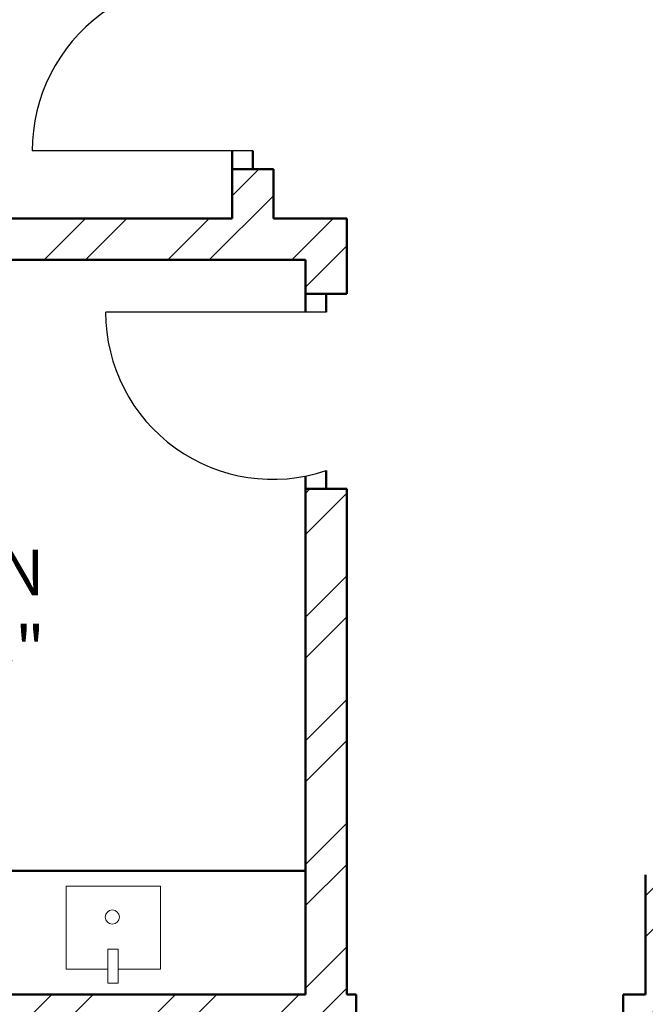
# Model space of a CAD drawing. Units: inches. Extents: x 1901 to 2863, y 888 to 2433.
# Tile 8 of 91: x 2086 to 2154, y 1442 to 1549. Entities that reach past the tile are written whole.
import ezdxf

# ---------------------------------------------------------------- set-up
doc = ezdxf.new("R2010")
doc.units = ezdxf.units.IN
for name, color, linetype, lineweight in [('A-AREA-IDEN', 7, 'Continuous', 18), ('A-DOOR', 4, 'Continuous', 25), ('A-FLOR-FIXT', 9, 'Continuous', 18), ('A-WALL', 7, 'Continuous', 50), ('A-WALL-PATT', 8, 'Continuous', 13)]:
    doc.layers.add(name, color=color, linetype=linetype, lineweight=lineweight)
doc.styles.get("Standard").update_dxf_attribs({"font": 'arial.ttf'})

msp = doc.modelspace()

# ---------------------------------------------------------------- hatches: boundary and pattern name
at = {"layer": 'A-WALL-PATT'}
h = msp.add_hatch(dxfattribs=at)
h.set_pattern_fill('ANSI32', color=256)
h.paths.add_polyline_path([(2192.5, 2274.13), (2141.26, 2274.13), (2141.26, 2269.63), (2192.5, 2269.63)])
h.paths.add_polyline_path([(2259.93, 2274.13), (2216.5, 2274.13), (2216.5, 2269.63), (2255.43, 2269.63), (2255.43, 2214.63), (2250.81, 2214.63), (2250.81, 2210.13), (2259.93, 2210.13), (2259.93, 2215.13), (2271.76, 2215.13), (2271.76, 2217.38), (2271.76, 2219.63), (2259.93, 2219.63)])
h.paths.add_polyline_path([(2171.43, 2269.63), (2166.93, 2269.63), (2166.93, 2219.63), (2121.24, 2219.63), (2121.24, 2215.13), (2166.93, 2215.13), (2166.93, 2083.13), (2161.81, 2083.13), (2161.81, 2078.63), (2171.43, 2078.63), (2177, 2078.63), (2177, 2080.88), (2177, 2083.13), (2171.43, 2083.13), (2171.43, 2210.13), (2230.91, 2210.13), (2230.91, 2212.38), (2230.91, 2214.63), (2171.43, 2214.63)])
h.paths.add_polyline_path([(2117.26, 2274.13), (2089.43, 2274.13), (2089.43, 2219.63), (2081.14, 2219.63), (2081.14, 2215.13), (2089.43, 2215.13), (2098, 2215.13), (2098, 2217.38), (2098, 2219.63), (2093.93, 2219.63), (2093.93, 2269.63), (2117.26, 2269.63), (2117.26, 2271.88)])
h.paths.add_polyline_path([(2343.43, 2219.63), (2329.29, 2219.63), (2329.29, 2215.13), (2338.93, 2215.13), (2338.93, 2184.74), (2343.43, 2184.74)])
h.paths.add_polyline_path([(2338.93, 2083.13), (2329.29, 2083.13), (2208.97, 2083.13), (2208.97, 2078.63), (2338.93, 2078.63)])
h.paths.add_polyline_path([(2343.43, 2136.74), (2338.93, 2136.74), (2338.93, 1872.63), (2343.43, 1872.63)])
h.paths.add_polyline_path([(2343.43, 1863.63), (2397.68, 1863.63), (2397.68, 1821.63), (2384.14, 1821.63), (2384.14, 1812.63), (2418.33, 1812.63), (2418.33, 1817.13), (2418.33, 1821.63), (2406.68, 1821.63), (2406.68, 1863.63), (2459.5, 1863.63), (2459.5, 1821.63), (2447.14, 1821.63), (2447.14, 1812.63), (2459.5, 1812.63), (2468.5, 1812.63), (2468.5, 1872.63), (2394.43, 1872.63), (2334.43, 1872.63), (2334.43, 1812.63), (2343.43, 1812.63), (2353.25, 1812.63), (2353.25, 1821.63), (2343.43, 1821.63)])
h.paths.add_polyline_path([(2510.01, 1872.63), (2468.5, 1872.63), (2468.5, 1868.13), (2510.01, 1868.13)])
h.paths.add_polyline_path([(2514.01, 1817.13), (2468.5, 1817.13), (2468.5, 1812.63), (2482.11, 1812.63), (2482.11, 1800.61), (2486.61, 1800.61), (2486.61, 1812.63), (2514.01, 1812.63)])
h.paths.add_polyline_path([(2299.25, 1814.88), (2299.25, 1817.13), (2295.93, 1817.13), (2295.93, 1854.17), (2293.68, 1854.17), (2291.43, 1854.17), (2291.43, 1817.13), (2266.11, 1817.13), (2266.11, 1812.63), (2299.25, 1812.63)])
h.paths.add_polyline_path([(2218.11, 1817.13), (2206.46, 1817.13), (2171.43, 1817.13), (2171.43, 1949.13), (2190.1, 1949.13), (2190.1, 1953.63), (2163.47, 1953.63), (2163.47, 1949.13), (2166.93, 1949.13), (2166.93, 1817.13), (2114.3, 1817.13), (2114.3, 1812.63), (2218.11, 1812.63)])
h.paths.add_polyline_path([(2029.43, 1970.92), (2024.93, 1970.92), (2024.93, 1912.72), (2029.43, 1912.72)])
h.paths.add_polyline_path([(2132.3, 1953.63), (2113.93, 1953.63), (2113.93, 1975.89), (2111.68, 1975.89), (2109.43, 1975.89), (2109.43, 1953.63), (2029.43, 1953.63), (2029.43, 1949.13), (2132.3, 1949.13)])
h.paths.add_polyline_path([(2029.43, 1853.61), (2029.31, 1853.61), (2029.31, 1853.61), (2029.43, 1853.61), (2029.43, 1864.72), (2024.93, 1864.72), (2024.93, 1812.63), (2066.3, 1812.63), (2066.3, 1814.88), (2066.3, 1817.13), (2029.43, 1817.13)])
h.paths.add_polyline_path([(2122.93, 2010.09), (2120.68, 2010.09), (2118.43, 2010.09), (2118.43, 2006.13), (2029.43, 2006.13), (2029.43, 2001.63), (2109.43, 2001.63), (2109.43, 1998.04), (2113.93, 1998.04), (2113.93, 2001.63), (2122.93, 2001.63)])
h.paths.add_polyline_path([(2029.43, 2031.38), (2024.93, 2031.38), (2024.93, 1994.92), (2027.18, 1994.92), (2029.43, 1994.92)])
h.paths.add_polyline_path([(2029.43, 2136.74), (2024.93, 2136.74), (2024.93, 2067.38), (2027.18, 2067.38), (2029.43, 2067.38)])
h.paths.add_polyline_path([(2125.62, 2083.13), (2029.43, 2083.13), (2029.43, 2078.63), (2118.43, 2078.63), (2118.43, 2030.71), (2122.93, 2030.71), (2122.93, 2078.63), (2125.62, 2078.63)])
h.paths.add_polyline_path([(2029.43, 2215.13), (2040.47, 2215.13), (2040.47, 2217.38), (2040.47, 2219.63), (2024.93, 2219.63), (2024.93, 2184.74), (2029.43, 2184.74), (2029.43, 2187.78)])
h.paths.add_polyline_path([(2686.43, 2274.13), (2659.28, 2274.13), (2659.28, 2269.63), (2681.93, 2269.63), (2681.93, 2219.63), (2676.82, 2219.63), (2676.82, 2215.13), (2681.93, 2215.13), (2697.01, 2215.13), (2697.01, 2217.38), (2697.01, 2219.63), (2686.43, 2219.63)])
h.paths.add_polyline_path([(2609.93, 2269.63), (2635.28, 2269.63), (2635.28, 2274.13), (2571.43, 2274.13), (2571.43, 2269.63), (2605.43, 2269.63), (2605.43, 2214.63), (2549.1, 2214.63), (2549.1, 2210.13), (2605.43, 2210.13), (2605.43, 2083.13), (2601.01, 2083.13), (2601.01, 2080.88), (2601.01, 2078.63), (2609.93, 2078.63), (2616.16, 2078.63), (2616.16, 2080.88), (2616.16, 2083.13), (2609.93, 2083.13), (2609.93, 2215.13), (2651.46, 2215.13), (2651.46, 2217.38), (2651.46, 2219.63), (2609.93, 2219.63)])
h.paths.add_polyline_path([(2521.43, 2269.63), (2547.43, 2269.63), (2547.43, 2271.88), (2547.43, 2274.13), (2516.93, 2274.13), (2516.93, 2219.63), (2506.41, 2219.63), (2506.41, 2215.13), (2516.93, 2215.13), (2516.93, 2210.13), (2525.4, 2210.13), (2525.4, 2212.38), (2525.4, 2214.63), (2521.43, 2214.63)])
h.paths.add_polyline_path([(2456.01, 2219.63), (2439.43, 2219.63), (2439.43, 2187.89), (2443.93, 2187.89), (2443.93, 2215.13), (2456.01, 2215.13)])
h.paths.add_polyline_path([(2752.93, 2219.63), (2739.48, 2219.63), (2739.48, 2215.13), (2748.43, 2215.13), (2748.43, 2187.89), (2752.93, 2187.89)])
h.paths.add_polyline_path([(2752.93, 2139.89), (2748.43, 2139.89), (2748.43, 2083.13), (2648.42, 2083.13), (2648.42, 2078.63), (2654.93, 2078.63), (2654.93, 2039.44), (2659.43, 2039.44), (2659.43, 2078.63), (2748.43, 2078.63), (2748.43, 2063.43), (2752.93, 2063.43)])
h.paths.add_polyline_path([(2752.93, 2010.63), (2659.43, 2010.63), (2659.43, 2015.65), (2654.93, 2015.65), (2654.93, 2010.63), (2605.43, 2010.63), (2605.43, 1920.97), (2609.93, 1920.97), (2609.93, 2006.13), (2748.43, 2006.13), (2748.43, 1982.47), (2752.93, 1982.47)])
h.paths.add_polyline_path([(2752.93, 2027.43), (2748.43, 2027.43), (2748.43, 2010.63), (2752.93, 2010.63)])
h.paths.add_polyline_path([(2748.43, 1886.13), (2609.93, 1886.13), (2609.93, 1889.72), (2605.43, 1889.72), (2605.43, 1861.26), (2609.93, 1861.26), (2609.93, 1881.63), (2748.43, 1881.63)])
h.paths.add_polyline_path([(2456.86, 2228.83), (2498.4, 2228.83), (2498.4, 2247.49), (2456.86, 2247.49)], flags=9)
h.paths.add_polyline_path([(2038.6, 2237.42), (2080.17, 2237.42), (2080.17, 2256.08), (2038.6, 2256.08)], flags=9)
h.paths.add_polyline_path([(2292.01, 1062.39), (2539.93, 1062.39), (2539.93, 1099.49), (2292.01, 1099.49)], flags=9)
h.paths.add_polyline_path([(2424.91, 1832.25), (2448.51, 1832.25), (2448.51, 1846.68), (2424.91, 1846.68)], flags=25)
h.paths.add_polyline_path([(2359.08, 1832.25), (2382.68, 1832.25), (2382.68, 1846.68), (2359.08, 1846.68)], flags=25)
h.paths.add_polyline_path([(2352.9, 1684.8), (2367.54, 1684.8), (2367.54, 1697.17), (2352.9, 1697.17)], flags=9)
h.paths.add_polyline_path([(2079.29, 1755.83), (2169.02, 1755.83), (2169.02, 1774.37), (2079.29, 1774.37)], flags=9)
h.paths.add_polyline_path([(2404.09, 1373.86), (2404.09, 1463.59), (2385.54, 1463.59), (2385.54, 1373.86)], flags=9)
h.paths.add_polyline_path([(2268.09, 2236.37), (2309.64, 2236.37), (2309.64, 2255.03), (2268.09, 2255.03)], flags=9)
h.paths.add_polyline_path([(2575.96, 1700.95), (2665.7, 1700.95), (2665.7, 1719.5), (2575.96, 1719.5)], flags=9)
h.paths.add_polyline_path([(2302.96, 1878.47), (2329.52, 1878.47), (2329.52, 1888.78), (2302.96, 1888.78)], flags=9)
h.paths.add_polyline_path([(2097.42, 2240.58), (2126.57, 2240.58), (2126.57, 2259.23), (2097.42, 2259.23)], flags=9)
h.paths.add_polyline_path([(2208.72, 2246.12), (2237.88, 2246.12), (2237.88, 2264.78), (2208.72, 2264.78)], flags=9)
h.paths.add_polyline_path([(2038.15, 1925.96), (2076.99, 1925.96), (2076.99, 1944.62), (2038.15, 1944.62)], flags=9)
h.paths.add_polyline_path([(2239.14, 1926.67), (2288.46, 1926.67), (2288.46, 1945.33), (2239.14, 1945.33)], flags=9)
h.paths.add_polyline_path([(2175.43, 2007.33), (2212.36, 2007.33), (2212.36, 2025.99), (2175.43, 2025.99)], flags=9)
h.paths.add_polyline_path([(2225.03, 2091.79), (2263.87, 2091.79), (2263.87, 2110.45), (2225.03, 2110.45)], flags=9)
h.paths.add_polyline_path([(2035.4, 2098.48), (2074.24, 2098.48), (2074.24, 2117.14), (2035.4, 2117.14)], flags=9)
h.paths.add_polyline_path([(2050.1, 2029.21), (2083.26, 2029.21), (2083.26, 2047.87), (2050.1, 2047.87)], flags=9)
h.paths.add_polyline_path([(2069.68, 1956.72), (2098.83, 1956.72), (2098.83, 1975.38), (2069.68, 1975.38)], flags=25)
h.paths.add_polyline_path([(2328.62, 1753.34), (2361.66, 1753.34), (2361.66, 1771.99), (2328.62, 1771.99)], flags=9)
h.paths.add_polyline_path([(2395.16, 2060.89), (2395.16, 2140.65), (2378.68, 2140.65), (2378.68, 2060.89)], flags=9)
h.paths.add_polyline_path([(2463.73, 2059.02), (2492.89, 2059.02), (2492.89, 2077.68), (2463.73, 2077.68)], flags=9)
h.paths.add_polyline_path([(2458.03, 2181.54), (2496.87, 2181.54), (2496.87, 2200.19), (2458.03, 2200.19)], flags=9)
h.paths.add_polyline_path([(2527.58, 2243.07), (2556.73, 2243.07), (2556.73, 2261.73), (2527.58, 2261.73)], flags=9)
h.paths.add_polyline_path([(2694.46, 2232.77), (2736.03, 2232.77), (2736.03, 2251.42), (2694.46, 2251.42)], flags=9)
h.paths.add_polyline_path([(2637.82, 2249.22), (2666.98, 2249.22), (2666.98, 2267.88), (2637.82, 2267.88)], flags=9)
h.paths.add_polyline_path([(2623.69, 2183.54), (2662.53, 2183.54), (2662.53, 2202.2), (2623.69, 2202.2)], flags=9)
h.paths.add_polyline_path([(2691.97, 2021.5), (2725.12, 2021.5), (2725.12, 2040.16), (2691.97, 2040.16)], flags=9)
h.paths.add_polyline_path([(2621.04, 1975.91), (2662.34, 1975.91), (2662.34, 1994.57), (2621.04, 1994.57)], flags=25)
h.paths.add_polyline_path([(2479.03, 1927.62), (2519.84, 1927.62), (2519.84, 1946.28), (2479.03, 1946.28)], flags=9)
h.paths.add_polyline_path([(2670.94, 1849.08), (2716.01, 1849.08), (2716.01, 1867.73), (2670.94, 1867.73)], flags=9)
h.paths.add_polyline_path([(2523.61, 1782.96), (2550.17, 1782.96), (2550.17, 1793.26), (2523.61, 1793.26)], flags=9)
h.paths.add_polyline_path([(2450.84, 1207.33), (2492.39, 1207.33), (2492.39, 1225.99), (2450.84, 1225.99)], flags=9)
h.paths.add_polyline_path([(2527.75, 1203.84), (2556.91, 1203.84), (2556.91, 1222.5), (2527.75, 1222.5)], flags=9)
h.paths.add_polyline_path([(2639.11, 1207.2), (2668.27, 1207.2), (2668.27, 1225.86), (2639.11, 1225.86)], flags=9)
h.paths.add_polyline_path([(2692.59, 1218.97), (2734.17, 1218.97), (2734.17, 1237.62), (2692.59, 1237.62)], flags=9)
h.paths.add_polyline_path([(2669.27, 1366.33), (2708.11, 1366.33), (2708.11, 1384.99), (2669.27, 1384.99)], flags=9)
h.paths.add_polyline_path([(2463.31, 1358.03), (2502.15, 1358.03), (2502.15, 1376.69), (2463.31, 1376.69)], flags=9)
h.paths.add_polyline_path([(2494.72, 1449.96), (2531.65, 1449.96), (2531.65, 1468.62), (2494.72, 1468.62)], flags=9)
h.paths.add_polyline_path([(2675.57, 1422.16), (2708.72, 1422.16), (2708.72, 1440.81), (2675.57, 1440.81)], flags=9)
h.paths.add_polyline_path([(2685.63, 1493.89), (2714.79, 1493.89), (2714.79, 1512.55), (2685.63, 1512.55)], flags=9)
h.paths.add_polyline_path([(2686.8, 1529.91), (2725.65, 1529.91), (2725.65, 1548.57), (2686.8, 1548.57)], flags=9)
h.paths.add_polyline_path([(2503.65, 1537.99), (2552.97, 1537.99), (2552.97, 1556.65), (2503.65, 1556.65)], flags=9)
h.paths.add_polyline_path([(2291.71, 1643.5), (2318.28, 1643.5), (2318.28, 1653.81), (2291.71, 1653.81)], flags=9)
h.paths.add_polyline_path([(2450.63, 1610.52), (2477.19, 1610.52), (2477.19, 1620.82), (2450.63, 1620.82)], flags=9)
h.paths.add_polyline_path([(2359.99, 1551.81), (2422.25, 1551.81), (2422.25, 1562.12), (2359.99, 1562.12)], flags=9)
h.paths.add_polyline_path([(2280.11, 1249.01), (2321.65, 1249.01), (2321.65, 1267.66), (2280.11, 1267.66)], flags=9)
h.paths.add_polyline_path([(2164.06, 1274.23), (2193.22, 1274.23), (2193.22, 1292.89), (2164.06, 1292.89)], flags=9)
h.paths.add_polyline_path([(2118.21, 1277.69), (2151.25, 1277.69), (2151.25, 1296.35), (2118.21, 1296.35)], flags=9)
h.paths.add_polyline_path([(2031.95, 1268.53), (2073.52, 1268.53), (2073.52, 1287.19), (2031.95, 1287.19)], flags=9)
h.paths.add_polyline_path([(2050.2, 1409.08), (2089.04, 1409.08), (2089.04, 1427.74), (2050.2, 1427.74)], flags=9)
h.paths.add_polyline_path([(2243.74, 1421.03), (2282.58, 1421.03), (2282.58, 1439.69), (2243.74, 1439.69)], flags=9)
h.paths.add_polyline_path([(2190.75, 1509.77), (2231.56, 1509.77), (2231.56, 1528.43), (2190.75, 1528.43)], flags=9)
h.paths.add_polyline_path([(2058.39, 1475.42), (2091.55, 1475.42), (2091.55, 1494.07), (2058.39, 1494.07)], flags=9)
h.paths.add_polyline_path([(2062.45, 1553.09), (2091.6, 1553.09), (2091.6, 1571.75), (2062.45, 1571.75)], flags=9)
h.paths.add_polyline_path([(2219.52, 1590.37), (2266.15, 1590.37), (2266.15, 1609.02), (2219.52, 1609.02)], flags=9)
h.paths.add_polyline_path([(2041.07, 1584.19), (2079.91, 1584.19), (2079.91, 1602.85), (2041.07, 1602.85)], flags=9)
h = msp.add_hatch(dxfattribs=at)
h.set_pattern_fill('ANSI32', color=256)
h.paths.add_polyline_path([(2443.93, 2139.89), (2439.43, 2139.89), (2439.43, 2069.35), (2441.68, 2069.35), (2443.93, 2069.35), (2443.93, 2078.63), (2521.93, 2078.63), (2521.93, 2075.07), (2524.18, 2075.07), (2526.43, 2075.07), (2526.43, 2078.63), (2571.75, 2078.63), (2571.75, 2080.88), (2571.75, 2083.13), (2443.93, 2083.13)])
h.paths.add_polyline_path([(2526.43, 2054.63), (2524.18, 2054.63), (2521.93, 2054.63), (2521.93, 2030.63), (2443.93, 2030.63), (2443.93, 2045.35), (2439.43, 2045.35), (2439.43, 1983.87), (2443.93, 1983.87), (2443.93, 2026.13), (2521.93, 2026.13), (2526.43, 2026.13)])
h.paths.add_polyline_path([(2443.93, 1923.87), (2439.43, 1923.87), (2439.43, 1872.63), (2443.93, 1872.63)])
h.paths.add_polyline_path([(2636.23, 1766.13), (2609.93, 1766.13), (2609.93, 1779.79), (2605.43, 1779.79), (2605.43, 1766.13), (2486.61, 1766.13), (2486.61, 1770.67), (2482.11, 1770.67), (2482.11, 1766.13), (2482.11, 1761.63), (2636.23, 1761.63), (2636.23, 1763.88)])
h.paths.add_polyline_path([(2519.54, 1663.38), (2519.54, 1665.63), (2494.93, 1665.63), (2481.83, 1665.63), (2481.83, 1663.38), (2481.83, 1661.13), (2490.43, 1661.13), (2490.43, 1640.16), (2494.93, 1640.16), (2494.93, 1661.13), (2519.54, 1661.13)])
h.paths.add_polyline_path([(2443.93, 1712.13), (2443.93, 1716.63), (2414.46, 1716.63), (2414.46, 1712.13), (2439.43, 1712.13), (2439.43, 1545.51), (2443.93, 1545.51), (2443.93, 1661.13), (2448.47, 1661.13), (2448.47, 1665.63), (2443.93, 1665.63)])
h.paths.add_polyline_path([(2343.43, 1712.13), (2365.52, 1712.13), (2365.52, 1714.38), (2365.52, 1716.63), (2333.87, 1716.63), (2333.87, 1714.38), (2333.87, 1712.13), (2338.93, 1712.13), (2338.93, 1575.63), (2338.93, 1545.51), (2343.43, 1545.51), (2343.43, 1547.51), (2343.43, 1580.13)])
h.paths.add_polyline_path([(2752.93, 1665.63), (2579.54, 1665.63), (2579.54, 1661.13), (2615.93, 1661.13), (2615.93, 1529.13), (2598.93, 1529.13), (2598.93, 1524.63), (2623.13, 1524.63), (2623.13, 1526.88), (2623.13, 1529.13), (2620.43, 1529.13), (2620.43, 1661.13), (2748.43, 1661.13), (2748.43, 1633.5), (2752.93, 1633.5)])
h.paths.add_polyline_path([(2752.93, 1419.93), (2748.43, 1419.93), (2748.43, 1400.13), (2659.43, 1400.13), (2659.43, 1444.33), (2657.18, 1444.33), (2654.93, 1444.33), (2654.93, 1400.13), (2643.65, 1400.13), (2643.65, 1395.63), (2748.43, 1395.63), (2748.43, 1364.04), (2752.93, 1364.04)])
h.paths.add_polyline_path([(2752.93, 1492.88), (2748.43, 1492.88), (2748.43, 1476.63), (2667.43, 1476.63), (2667.43, 1479.71), (2665.18, 1479.71), (2662.93, 1479.71), (2662.93, 1476.63), (2654.93, 1476.63), (2654.93, 1469.54), (2659.43, 1469.54), (2659.43, 1472.13), (2748.43, 1472.13), (2748.43, 1455.93), (2752.93, 1455.93)])
h.paths.add_polyline_path([(2752.93, 1304.04), (2748.43, 1304.04), (2748.43, 1263.63), (2738.66, 1263.63), (2738.66, 1259.13), (2752.93, 1259.13)])
h.paths.add_polyline_path([(2685.93, 1259.13), (2695.49, 1259.13), (2695.49, 1261.38), (2695.49, 1263.63), (2677.84, 1263.63), (2677.84, 1261.38), (2677.84, 1259.13), (2681.43, 1259.13), (2681.43, 1203.63), (2653.28, 1203.63), (2653.28, 1199.13), (2685.93, 1199.13), (2685.93, 1203.63)])
h.paths.add_polyline_path([(2609.43, 1395.63), (2611.85, 1395.63), (2611.85, 1400.13), (2598.89, 1400.13), (2598.89, 1397.88), (2598.89, 1395.63), (2604.93, 1395.63), (2604.93, 1268.13), (2554.73, 1268.13), (2554.73, 1265.88), (2554.73, 1263.63), (2604.93, 1263.63), (2604.93, 1203.63), (2571.31, 1203.63), (2571.31, 1199.13), (2604.93, 1199.13), (2629.28, 1199.13), (2629.28, 1201.38), (2629.28, 1203.63), (2609.43, 1203.63), (2609.43, 1258.63), (2609.43, 1259.13), (2654.8, 1259.13), (2654.8, 1263.63), (2609.43, 1263.63)])
h.paths.add_polyline_path([(2443.93, 1304.04), (2439.43, 1304.04), (2439.43, 1259.13), (2443.93, 1259.13), (2456.16, 1259.13), (2456.16, 1261.38), (2456.16, 1263.63), (2443.93, 1263.63)])
h.paths.add_polyline_path([(2525.43, 1263.63), (2531.78, 1263.63), (2531.78, 1268.13), (2520.93, 1268.13), (2520.93, 1263.63), (2511.41, 1263.63), (2511.41, 1259.13), (2520.93, 1259.13), (2520.93, 1199.13), (2547.31, 1199.13), (2547.31, 1201.38), (2547.31, 1203.63), (2525.43, 1203.63)])
h.paths.add_polyline_path([(2443.93, 1434.84), (2439.43, 1434.84), (2439.43, 1364.04), (2441.68, 1364.04), (2443.93, 1364.04)])
h.paths.add_polyline_path([(2567.13, 1400.13), (2443.93, 1400.13), (2443.93, 1395.63), (2567.13, 1395.63)])
h.paths.add_polyline_path([(2443.93, 1545.51), (2439.43, 1545.51), (2439.43, 1494.84), (2443.93, 1494.84)])
h.paths.add_polyline_path([(2494.93, 1553.35), (2492.68, 1553.35), (2490.43, 1553.35), (2490.43, 1524.63), (2494.93, 1524.63), (2525.94, 1524.63), (2525.94, 1526.88), (2525.94, 1529.13), (2494.93, 1529.13)])
h.paths.add_polyline_path([(2752.93, 1573.5), (2748.43, 1573.5), (2748.43, 1529.13), (2657.76, 1529.13), (2657.76, 1524.63), (2662.93, 1524.63), (2662.93, 1498.63), (2667.43, 1498.63), (2667.43, 1524.63), (2748.43, 1524.63), (2748.43, 1516.88), (2752.93, 1516.88)])
h.paths.add_polyline_path([(2038.6, 2237.42), (2080.17, 2237.42), (2080.17, 2256.08), (2038.6, 2256.08)], flags=9)
h.paths.add_polyline_path([(2292.01, 1062.39), (2539.93, 1062.39), (2539.93, 1099.49), (2292.01, 1099.49)], flags=9)
h.paths.add_polyline_path([(2424.91, 1832.25), (2448.51, 1832.25), (2448.51, 1846.68), (2424.91, 1846.68)], flags=9)
h.paths.add_polyline_path([(2359.08, 1832.25), (2382.68, 1832.25), (2382.68, 1846.68), (2359.08, 1846.68)], flags=9)
h.paths.add_polyline_path([(2352.9, 1684.8), (2367.54, 1684.8), (2367.54, 1697.17), (2352.9, 1697.17)], flags=9)
h.paths.add_polyline_path([(2079.29, 1755.83), (2169.02, 1755.83), (2169.02, 1774.37), (2079.29, 1774.37)], flags=9)
h.paths.add_polyline_path([(2404.09, 1373.86), (2404.09, 1463.59), (2385.54, 1463.59), (2385.54, 1373.86)], flags=9)
h.paths.add_polyline_path([(2268.09, 2236.37), (2309.64, 2236.37), (2309.64, 2255.03), (2268.09, 2255.03)], flags=9)
h.paths.add_polyline_path([(2575.96, 1700.95), (2665.7, 1700.95), (2665.7, 1719.5), (2575.96, 1719.5)], flags=9)
h.paths.add_polyline_path([(2302.96, 1878.47), (2329.52, 1878.47), (2329.52, 1888.78), (2302.96, 1888.78)], flags=9)
h.paths.add_polyline_path([(2097.42, 2240.58), (2126.57, 2240.58), (2126.57, 2259.23), (2097.42, 2259.23)], flags=9)
h.paths.add_polyline_path([(2208.72, 2246.12), (2237.88, 2246.12), (2237.88, 2264.78), (2208.72, 2264.78)], flags=9)
h.paths.add_polyline_path([(2038.15, 1925.96), (2076.99, 1925.96), (2076.99, 1944.62), (2038.15, 1944.62)], flags=9)
h.paths.add_polyline_path([(2239.14, 1926.67), (2288.46, 1926.67), (2288.46, 1945.33), (2239.14, 1945.33)], flags=9)
h.paths.add_polyline_path([(2175.43, 2007.33), (2212.36, 2007.33), (2212.36, 2025.99), (2175.43, 2025.99)], flags=9)
h.paths.add_polyline_path([(2225.03, 2091.79), (2263.87, 2091.79), (2263.87, 2110.45), (2225.03, 2110.45)], flags=9)
h.paths.add_polyline_path([(2035.4, 2098.48), (2074.24, 2098.48), (2074.24, 2117.14), (2035.4, 2117.14)], flags=9)
h.paths.add_polyline_path([(2050.1, 2029.21), (2083.26, 2029.21), (2083.26, 2047.87), (2050.1, 2047.87)], flags=9)
h.paths.add_polyline_path([(2069.68, 1956.72), (2098.83, 1956.72), (2098.83, 1975.38), (2069.68, 1975.38)], flags=9)
h.paths.add_polyline_path([(2328.62, 1753.34), (2361.66, 1753.34), (2361.66, 1771.99), (2328.62, 1771.99)], flags=9)
h.paths.add_polyline_path([(2395.16, 2060.89), (2395.16, 2140.65), (2378.68, 2140.65), (2378.68, 2060.89)], flags=9)
h.paths.add_polyline_path([(2463.73, 2059.02), (2492.89, 2059.02), (2492.89, 2077.68), (2463.73, 2077.68)], flags=9)
h.paths.add_polyline_path([(2458.03, 2181.54), (2496.87, 2181.54), (2496.87, 2200.19), (2458.03, 2200.19)], flags=9)
h.paths.add_polyline_path([(2456.86, 2228.83), (2498.4, 2228.83), (2498.4, 2247.49), (2456.86, 2247.49)], flags=9)
h.paths.add_polyline_path([(2527.58, 2243.07), (2556.73, 2243.07), (2556.73, 2261.73), (2527.58, 2261.73)], flags=9)
h.paths.add_polyline_path([(2694.46, 2232.77), (2736.03, 2232.77), (2736.03, 2251.42), (2694.46, 2251.42)], flags=9)
h.paths.add_polyline_path([(2637.82, 2249.22), (2666.98, 2249.22), (2666.98, 2267.88), (2637.82, 2267.88)], flags=9)
h.paths.add_polyline_path([(2623.69, 2183.54), (2662.53, 2183.54), (2662.53, 2202.2), (2623.69, 2202.2)], flags=9)
h.paths.add_polyline_path([(2691.97, 2021.5), (2725.12, 2021.5), (2725.12, 2040.16), (2691.97, 2040.16)], flags=9)
h.paths.add_polyline_path([(2621.04, 1975.91), (2662.34, 1975.91), (2662.34, 1994.57), (2621.04, 1994.57)], flags=9)
h.paths.add_polyline_path([(2479.03, 1927.62), (2519.84, 1927.62), (2519.84, 1946.28), (2479.03, 1946.28)], flags=9)
h.paths.add_polyline_path([(2670.94, 1849.08), (2716.01, 1849.08), (2716.01, 1867.73), (2670.94, 1867.73)], flags=9)
h.paths.add_polyline_path([(2523.61, 1782.96), (2550.17, 1782.96), (2550.17, 1793.26), (2523.61, 1793.26)], flags=9)
h.paths.add_polyline_path([(2450.84, 1207.33), (2492.39, 1207.33), (2492.39, 1225.99), (2450.84, 1225.99)], flags=9)
h.paths.add_polyline_path([(2527.75, 1203.84), (2556.91, 1203.84), (2556.91, 1222.5), (2527.75, 1222.5)], flags=9)
h.paths.add_polyline_path([(2639.11, 1207.2), (2668.27, 1207.2), (2668.27, 1225.86), (2639.11, 1225.86)], flags=9)
h.paths.add_polyline_path([(2692.59, 1218.97), (2734.17, 1218.97), (2734.17, 1237.62), (2692.59, 1237.62)], flags=9)
h.paths.add_polyline_path([(2669.27, 1366.33), (2708.11, 1366.33), (2708.11, 1384.99), (2669.27, 1384.99)], flags=25)
h.paths.add_polyline_path([(2463.31, 1358.03), (2502.15, 1358.03), (2502.15, 1376.69), (2463.31, 1376.69)], flags=9)
h.paths.add_polyline_path([(2494.72, 1449.96), (2531.65, 1449.96), (2531.65, 1468.62), (2494.72, 1468.62)], flags=9)
h.paths.add_polyline_path([(2675.57, 1422.16), (2708.72, 1422.16), (2708.72, 1440.81), (2675.57, 1440.81)], flags=25)
h.paths.add_polyline_path([(2685.63, 1493.89), (2714.79, 1493.89), (2714.79, 1512.55), (2685.63, 1512.55)], flags=9)
h.paths.add_polyline_path([(2686.8, 1529.91), (2725.65, 1529.91), (2725.65, 1548.57), (2686.8, 1548.57)], flags=25)
h.paths.add_polyline_path([(2503.65, 1537.99), (2552.97, 1537.99), (2552.97, 1556.65), (2503.65, 1556.65)], flags=9)
h.paths.add_polyline_path([(2291.71, 1643.5), (2318.28, 1643.5), (2318.28, 1653.81), (2291.71, 1653.81)], flags=9)
h.paths.add_polyline_path([(2450.63, 1610.52), (2477.19, 1610.52), (2477.19, 1620.82), (2450.63, 1620.82)], flags=9)
h.paths.add_polyline_path([(2359.99, 1551.81), (2422.25, 1551.81), (2422.25, 1562.12), (2359.99, 1562.12)], flags=9)
h.paths.add_polyline_path([(2280.11, 1249.01), (2321.65, 1249.01), (2321.65, 1267.66), (2280.11, 1267.66)], flags=9)
h.paths.add_polyline_path([(2164.06, 1274.23), (2193.22, 1274.23), (2193.22, 1292.89), (2164.06, 1292.89)], flags=9)
h.paths.add_polyline_path([(2118.21, 1277.69), (2151.25, 1277.69), (2151.25, 1296.35), (2118.21, 1296.35)], flags=9)
h.paths.add_polyline_path([(2031.95, 1268.53), (2073.52, 1268.53), (2073.52, 1287.19), (2031.95, 1287.19)], flags=9)
h.paths.add_polyline_path([(2050.2, 1409.08), (2089.04, 1409.08), (2089.04, 1427.74), (2050.2, 1427.74)], flags=9)
h.paths.add_polyline_path([(2243.74, 1421.03), (2282.58, 1421.03), (2282.58, 1439.69), (2243.74, 1439.69)], flags=9)
h.paths.add_polyline_path([(2190.75, 1509.77), (2231.56, 1509.77), (2231.56, 1528.43), (2190.75, 1528.43)], flags=9)
h.paths.add_polyline_path([(2058.39, 1475.42), (2091.55, 1475.42), (2091.55, 1494.07), (2058.39, 1494.07)], flags=9)
h.paths.add_polyline_path([(2062.45, 1553.09), (2091.6, 1553.09), (2091.6, 1571.75), (2062.45, 1571.75)], flags=9)
h.paths.add_polyline_path([(2219.52, 1590.37), (2266.15, 1590.37), (2266.15, 1609.02), (2219.52, 1609.02)], flags=9)
h.paths.add_polyline_path([(2041.07, 1584.19), (2079.91, 1584.19), (2079.91, 1602.85), (2041.07, 1602.85)], flags=9)
h = msp.add_hatch(dxfattribs=at)
h.set_pattern_fill('ANSI32', color=256)
h.paths.add_polyline_path([(2182.93, 1716.63), (2024.93, 1716.63), (2024.93, 1681.7), (2029.33, 1681.7), (2029.33, 1712.13), (2154.33, 1712.13), (2154.33, 1580.13), (2148.52, 1580.13), (2148.52, 1577.88), (2148.52, 1575.63), (2194.93, 1575.63), (2194.93, 1580.13), (2158.83, 1580.13), (2158.83, 1712.13), (2182.93, 1712.13)])
h.paths.add_polyline_path([(2301.07, 1716.63), (2242.93, 1716.63), (2242.93, 1712.13), (2283.83, 1712.13), (2283.83, 1685.54), (2288.33, 1685.54), (2288.33, 1712.13), (2301.07, 1712.13)])
h.paths.add_polyline_path([(2288.33, 1600.41), (2286.08, 1600.41), (2283.83, 1600.41), (2283.83, 1580.13), (2270.6, 1580.13), (2270.6, 1575.63), (2288.33, 1575.63)])
h.paths.add_polyline_path([(2295.93, 1953.63), (2271.45, 1953.63), (2271.45, 1949.13), (2291.43, 1949.13), (2291.43, 1941.24), (2295.93, 1941.24)])
h.paths.add_polyline_path([(2098.38, 1244.13), (2082.33, 1244.13), (2082.33, 1302.13), (2086.52, 1302.13), (2086.52, 1306.63), (2067.46, 1306.63), (2067.46, 1302.13), (2077.83, 1302.13), (2077.83, 1239.63), (2098.38, 1239.63), (2098.38, 1241.88)])
h.paths.add_polyline_path([(2217.31, 1306.63), (2158.83, 1306.63), (2158.83, 1451.63), (2162.72, 1451.63), (2162.72, 1453.88), (2162.72, 1456.13), (2154.33, 1456.13), (2154.33, 1443.13), (2151.91, 1443.13), (2151.91, 1438.63), (2154.33, 1438.63), (2154.33, 1306.63), (2109.31, 1306.63), (2109.31, 1304.38), (2109.31, 1302.13), (2154.33, 1302.13), (2154.33, 1244.13), (2122.38, 1244.13), (2122.38, 1239.63), (2154.33, 1239.63), (2154.33, 1223.63), (2163.33, 1223.63), (2181.01, 1223.63), (2181.01, 1225.88), (2181.01, 1228.13), (2163.33, 1228.13), (2163.33, 1258.22), (2158.83, 1258.22), (2158.83, 1302.13), (2217.31, 1302.13)])
h.paths.add_polyline_path([(2259.99, 1306.63), (2238.3, 1306.63), (2238.3, 1304.38), (2238.3, 1302.13), (2242.83, 1302.13), (2242.83, 1228.13), (2205.01, 1228.13), (2205.01, 1223.63), (2247.33, 1223.63), (2247.33, 1302.13), (2259.99, 1302.13), (2259.99, 1304.38)])
h.paths.add_polyline_path([(2343.43, 1361.7), (2338.93, 1361.7), (2338.93, 1306.63), (2322.38, 1306.63), (2322.38, 1302.13), (2343.43, 1302.13)])
h.paths.add_polyline_path([(2343.43, 1470.4), (2338.93, 1470.4), (2338.93, 1456.13), (2193.73, 1456.13), (2193.73, 1453.88), (2193.73, 1451.63), (2338.93, 1451.63), (2338.93, 1421.7), (2343.43, 1421.7)])
h.paths.add_polyline_path([(2343.43, 1545.51), (2338.93, 1545.51), (2338.93, 1530.4), (2343.43, 1530.4)])
h.paths.add_polyline_path([(2029.33, 1466.83), (2024.93, 1466.83), (2024.93, 1409.82), (2029.33, 1409.82)])
h.paths.add_polyline_path([(2122.84, 1440.88), (2122.84, 1443.13), (2121.83, 1443.13), (2121.83, 1498.18), (2119.58, 1498.18), (2117.33, 1498.18), (2117.33, 1443.13), (2029.33, 1443.13), (2029.33, 1438.63), (2122.84, 1438.63)])
h.paths.add_polyline_path([(2029.33, 1543.05), (2024.93, 1543.05), (2024.93, 1502.83), (2029.33, 1502.83)])
h.paths.add_polyline_path([(2029.33, 1621.7), (2024.93, 1621.7), (2024.93, 1567.05), (2027.13, 1567.05), (2029.33, 1567.05), (2029.33, 1575.63), (2109.33, 1575.63), (2109.33, 1554.71), (2113.83, 1554.71), (2113.83, 1575.63), (2115.8, 1575.63), (2115.8, 1577.88), (2115.8, 1580.13), (2029.33, 1580.13)])
h.paths.add_polyline_path([(2121.83, 1527.63), (2117.33, 1527.63), (2113.83, 1527.63), (2113.83, 1533.01), (2111.58, 1533.01), (2109.33, 1533.01), (2109.33, 1527.63), (2029.33, 1527.63), (2029.33, 1523.13), (2117.33, 1523.13), (2117.33, 1519.43), (2121.83, 1519.43)])
h.paths.add_polyline_path([(2029.33, 1349.82), (2024.93, 1349.82), (2024.93, 1302.13), (2036.28, 1302.13), (2036.28, 1306.63), (2029.33, 1306.63)])

# ---------------------------------------------------------------- linework, layer by layer
at = {"layer": 'A-DOOR'}
for p, q in [((2111.58, 1535.01), (2087.58, 1535.01)), ((2119.58, 1517.43), (2095.58, 1517.43))]:
    msp.add_line(p, q, dxfattribs=at)
for centre, radius, start, end in [((2106.11, 1535.01), 18.53, 72.8301, 180), ((2113.77, 1517.43), 18.2, 180, 288.5945)]:
    msp.add_arc(centre, radius, start, end, dxfattribs=at)
at = {"layer": 'A-FLOR-FIXT'}
msp.add_lwpolyline([(2096.94, 1445.87), (2101.53, 1445.87), (2101.53, 1454.92), (2091.26, 1454.92), (2091.26, 1445.87), (2095.81, 1445.87)], dxfattribs=at)
msp.add_lwpolyline([(2095.81, 1444.34), (2096.94, 1444.34), (2096.94, 1448.04), (2095.81, 1448.04)], close=True, dxfattribs=at)
msp.add_circle((2096.3, 1451.55), 0.768, dxfattribs=at)
at = {"layer": 'A-WALL'}
for p, q in [((2109.33, 1535.01), (2109.33, 1527.63)), ((2111.58, 1533.01), (2111.58, 1535.01)), ((2109.33, 1533.01), (2113.83, 1533.01)), ((2113.83, 1533.01), (2111.58, 1533.01)), ((2113.83, 1527.63), (2113.83, 1533.01)), ((2109.33, 1527.63), (2029.33, 1527.63)), ((2113.83, 1527.63), (2117.33, 1527.63)), ((2121.83, 1527.63), (2117.33, 1527.63)), ((2121.83, 1519.43), (2121.83, 1527.63)), ((2117.33, 1523.13), (2029.33, 1523.13)), ((2117.33, 1523.13), (2117.33, 1517.43)), ((2117.33, 1519.43), (2121.83, 1519.43)), ((2121.83, 1519.43), (2119.58, 1519.43)), ((2119.58, 1519.43), (2119.58, 1517.43)), ((2117.33, 1499.58), (2117.33, 1443.13)), ((2119.58, 1498.18), (2119.58, 1500.18)), ((2117.33, 1498.18), (2121.83, 1498.18)), ((2121.83, 1498.18), (2119.58, 1498.18)), ((2121.83, 1443.13), (2121.83, 1498.18)), ((2117.33, 1456.6), (2043.06, 1456.6)), ((2154.33, 1456.13), (2154.33, 1443.13)), ((2117.33, 1443.13), (2029.33, 1443.13)), ((2122.84, 1443.13), (2121.83, 1443.13)), ((2122.84, 1443.13), (2122.84, 1438.63)), ((2154.33, 1443.13), (2151.91, 1443.13)), ((2151.91, 1443.13), (2151.91, 1438.63))]:
    msp.add_line(p, q, dxfattribs=at)

# ---------------------------------------------------------------- texts
at = {"layer": 'A-AREA-IDEN', "insert": (2060.15, 1491.58), "char_height": 5, "attachment_point": 1}
msp.add_mtext_dynamic_manual_height_columns('KITCHEN\\P7\'4"x6\'8"', width=173.0579, gutter_width=12.5, heights=[0], dxfattribs=at)

doc.saveas('drawing.dxf')
